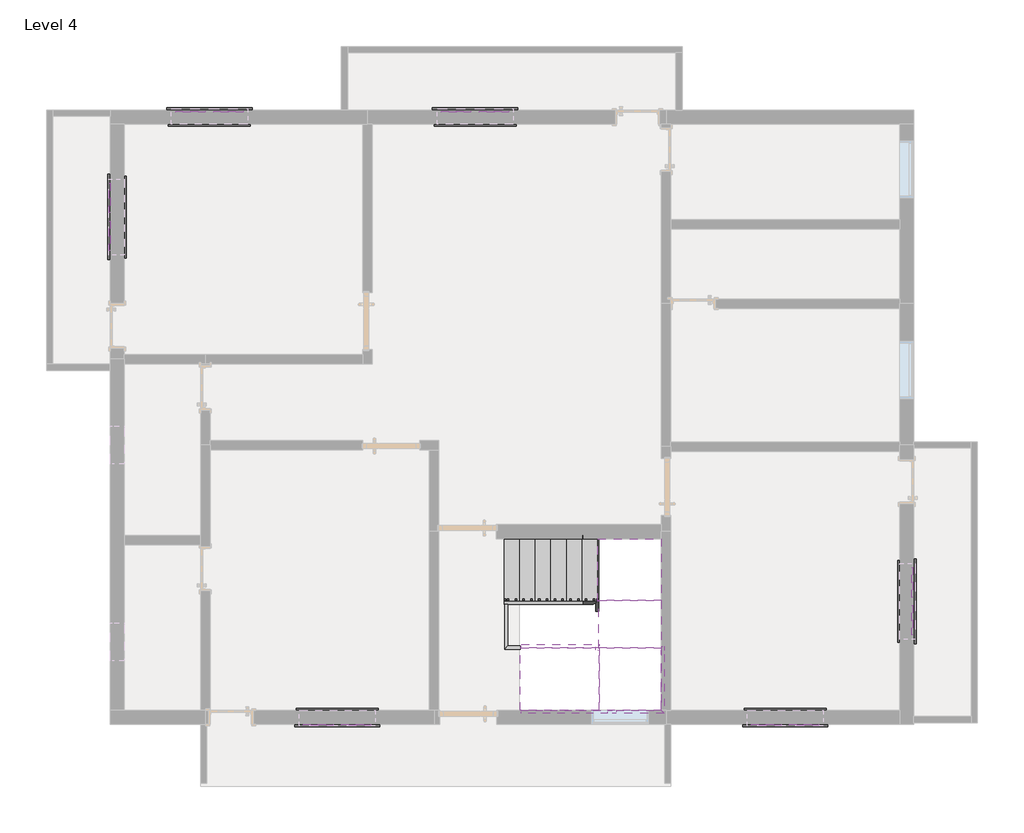
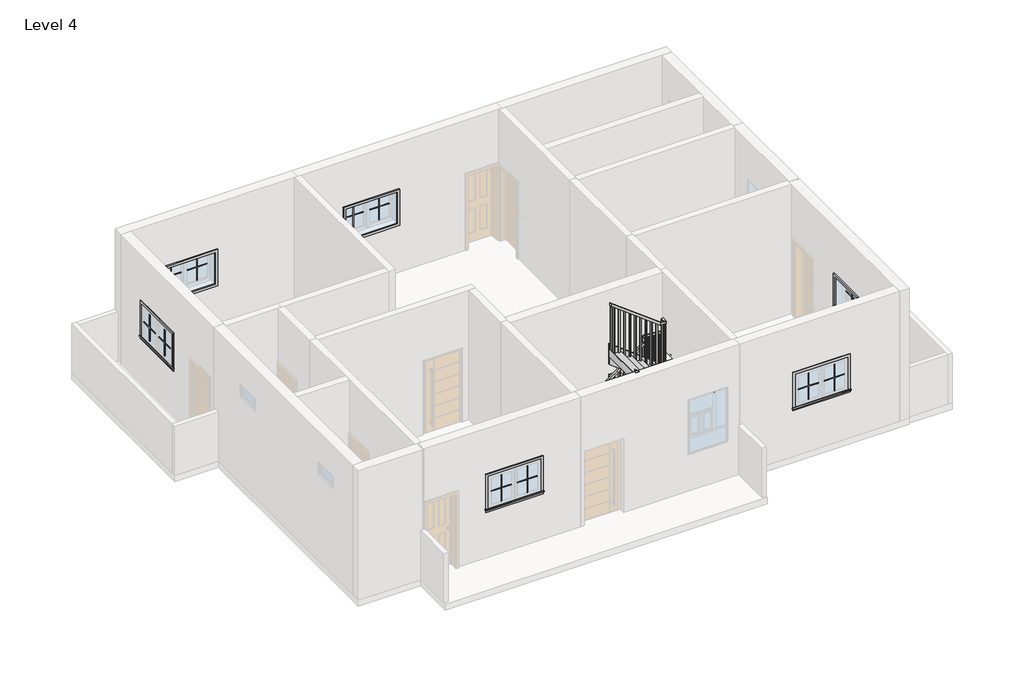
# One storey, part 3 of 3: 24 proxies, 11 members, 3 stair flights, 2 railings, 2 slabs.
"""IFC4 building model written with IfcOpenShell, lengths in millimetres."""

from ifc_helpers import new_model, si_unit, frame, origin, place, context, project, spatial, polyline, outline, extrude, faceted_brep, transform, mapped, element, save
from components import m_muntin_pattern_2x2_m_muntin_pattern_2x2_8d9e5da3, m_muntin_pattern_2x2_m_muntin_pattern_2x2_32a0f80e, m_trim_window_exterior_flat_with_sill_3a557199, m_trim_window_interior_flat_picture_frame_580345df, non_monolithic_landing_cef648f3, non_monolithic_landing_62522cc9, stair_flight_50mm_tread_13mm_riser_d6021486, stair_flight_50mm_tread_13mm_riser_ddd89fd2, stair_flight_50mm_tread_13mm_riser_ab5ce904

model = new_model("IFC4")

# Units and contexts
model_context = context("Model", 3, world=origin())
ifc_project = project(units=[si_unit("LENGTHUNIT", "METRE", prefix="MILLI")], contexts=[model_context])

# Site, building, storey
site = spatial("IfcSite", under=ifc_project)
building = spatial("IfcBuilding", under=site)
storey = spatial("IfcBuildingStorey", under=building, Name="Level 4", Elevation=9601.2)

# Proxies
placement = place(None, origin())
m_muntin_pattern_2x2_m_muntin_pattern_2x2_shape = m_muntin_pattern_2x2_m_muntin_pattern_2x2_8d9e5da3(model_context)
element("IfcBuildingElementProxy", 1, Name="M_Muntin Pattern_2x2 : M_Muntin Pattern_2x2", ObjectType="M_Muntin Pattern_2x2 : M_Muntin Pattern_2x2", at=placement, inside=storey, context=model_context, shape_type="MappedRepresentation", body=[
    mapped(m_muntin_pattern_2x2_m_muntin_pattern_2x2_shape, transform((-14356.7669909, -4470.2368509, 10890.25), x_axis=(-1.0, 0.0, 0.0), y_axis=(0.0, -1.0, 0.0), z_axis=(0.0, 0.0, 1.0))),
])
element("IfcBuildingElementProxy", 2, Name="M_Muntin Pattern_2x2 : M_Muntin Pattern_2x2", ObjectType="M_Muntin Pattern_2x2 : M_Muntin Pattern_2x2", at=placement, inside=storey, context=model_context, shape_type="MappedRepresentation", body=[
    mapped(m_muntin_pattern_2x2_m_muntin_pattern_2x2_shape, transform((-17007.0919909, 5340.5131491, 10890.25), x_axis=(1.0, 0.0, 0.0), y_axis=(0.0, 1.0, 0.0), z_axis=(0.0, 0.0, 1.0))),
])
element("IfcBuildingElementProxy", 3, Name="M_Muntin Pattern_2x2 : M_Muntin Pattern_2x2", ObjectType="M_Muntin Pattern_2x2 : M_Muntin Pattern_2x2", at=placement, inside=storey, context=model_context, shape_type="MappedRepresentation", body=[
    mapped(m_muntin_pattern_2x2_m_muntin_pattern_2x2_shape, transform((-18281.8544909, 3334.7006491, 10890.25), x_axis=(0.0, 1.0, 0.0), y_axis=(-1.0, 0.0, 0.0), z_axis=(0.0, 0.0, 1.0))),
])
element("IfcBuildingElementProxy", 4, Name="M_Muntin Pattern_2x2 : M_Muntin Pattern_2x2", ObjectType="M_Muntin Pattern_2x2 : M_Muntin Pattern_2x2", at=placement, inside=storey, context=model_context, shape_type="MappedRepresentation", body=[
    mapped(m_muntin_pattern_2x2_m_muntin_pattern_2x2_shape, transform((-12757.3544909, 5340.5131491, 10890.25), x_axis=(1.0, 0.0, 0.0), y_axis=(0.0, 1.0, 0.0), z_axis=(0.0, 0.0, 1.0))),
])
element("IfcBuildingElementProxy", 5, Name="M_Muntin Pattern_2x2 : M_Muntin Pattern_2x2", ObjectType="M_Muntin Pattern_2x2 : M_Muntin Pattern_2x2", at=placement, inside=storey, context=model_context, shape_type="MappedRepresentation", body=[
    mapped(m_muntin_pattern_2x2_m_muntin_pattern_2x2_shape, transform((-5448.5044909, -2207.2493509, 10890.25), x_axis=(0.0, -1.0, 0.0), y_axis=(1.0, 0.0, 0.0), z_axis=(0.0, 0.0, 1.0))),
])
element("IfcBuildingElementProxy", 6, Name="M_Muntin Pattern_2x2 : M_Muntin Pattern_2x2", ObjectType="M_Muntin Pattern_2x2 : M_Muntin Pattern_2x2", at=placement, inside=storey, context=model_context, shape_type="MappedRepresentation", body=[
    mapped(m_muntin_pattern_2x2_m_muntin_pattern_2x2_shape, transform((-7193.1669909, -4470.2368509, 10890.25), x_axis=(-1.0, 0.0, 0.0), y_axis=(0.0, -1.0, 0.0), z_axis=(0.0, 0.0, 1.0))),
])
m_muntin_pattern_2x2_m_muntin_pattern_2x2_2_shape = m_muntin_pattern_2x2_m_muntin_pattern_2x2_32a0f80e(model_context)
element("IfcBuildingElementProxy", 7, Name="M_Muntin Pattern_2x2 : M_Muntin Pattern_2x2", ObjectType="M_Muntin Pattern_2x2 : M_Muntin Pattern_2x2", at=placement, inside=storey, context=model_context, shape_type="MappedRepresentation", body=[
    mapped(m_muntin_pattern_2x2_m_muntin_pattern_2x2_2_shape, transform((-14963.1919909, -4470.2368509, 10890.25), x_axis=(1.0, 0.0, 0.0), y_axis=(0.0, 1.0, 0.0), z_axis=(0.0, 0.0, 1.0))),
])
element("IfcBuildingElementProxy", 8, Name="M_Muntin Pattern_2x2 : M_Muntin Pattern_2x2", ObjectType="M_Muntin Pattern_2x2 : M_Muntin Pattern_2x2", at=placement, inside=storey, context=model_context, shape_type="MappedRepresentation", body=[
    mapped(m_muntin_pattern_2x2_m_muntin_pattern_2x2_2_shape, transform((-16400.6669909, 5340.5131491, 10890.25), x_axis=(-1.0, 0.0, 0.0), y_axis=(0.0, -1.0, 0.0), z_axis=(0.0, 0.0, 1.0))),
])
element("IfcBuildingElementProxy", 9, Name="M_Muntin Pattern_2x2 : M_Muntin Pattern_2x2", ObjectType="M_Muntin Pattern_2x2 : M_Muntin Pattern_2x2", at=placement, inside=storey, context=model_context, shape_type="MappedRepresentation", body=[
    mapped(m_muntin_pattern_2x2_m_muntin_pattern_2x2_2_shape, transform((-18281.8544909, 3941.1256491, 10890.25), x_axis=(0.0, -1.0, 0.0), y_axis=(1.0, 0.0, 0.0), z_axis=(0.0, 0.0, 1.0))),
])
element("IfcBuildingElementProxy", 10, Name="M_Muntin Pattern_2x2 : M_Muntin Pattern_2x2", ObjectType="M_Muntin Pattern_2x2 : M_Muntin Pattern_2x2", at=placement, inside=storey, context=model_context, shape_type="MappedRepresentation", body=[
    mapped(m_muntin_pattern_2x2_m_muntin_pattern_2x2_2_shape, transform((-12150.9294909, 5340.5131491, 10890.25), x_axis=(-1.0, 0.0, 0.0), y_axis=(0.0, -1.0, 0.0), z_axis=(0.0, 0.0, 1.0))),
])
element("IfcBuildingElementProxy", 11, Name="M_Muntin Pattern_2x2 : M_Muntin Pattern_2x2", ObjectType="M_Muntin Pattern_2x2 : M_Muntin Pattern_2x2", at=placement, inside=storey, context=model_context, shape_type="MappedRepresentation", body=[
    mapped(m_muntin_pattern_2x2_m_muntin_pattern_2x2_2_shape, transform((-5448.5044909, -2813.6743509, 10890.25), x_axis=(0.0, 1.0, 0.0), y_axis=(-1.0, 0.0, 0.0), z_axis=(0.0, 0.0, 1.0))),
])
element("IfcBuildingElementProxy", 12, Name="M_Muntin Pattern_2x2 : M_Muntin Pattern_2x2", ObjectType="M_Muntin Pattern_2x2 : M_Muntin Pattern_2x2", at=placement, inside=storey, context=model_context, shape_type="MappedRepresentation", body=[
    mapped(m_muntin_pattern_2x2_m_muntin_pattern_2x2_2_shape, transform((-7799.5919909, -4470.2368509, 10890.25), x_axis=(1.0, 0.0, 0.0), y_axis=(0.0, 1.0, 0.0), z_axis=(0.0, 0.0, 1.0))),
])
m_trim_window_exterior_flat_with_sill_shape = m_trim_window_exterior_flat_with_sill_3a557199(model_context)
element("IfcBuildingElementProxy", 13, Name="M_Trim-Window-Exterior-Flat : with Sill", ObjectType="M_Trim-Window-Exterior-Flat : with Sill", at=placement, inside=storey, context=model_context, shape_type="MappedRepresentation", body=[
    mapped(m_trim_window_exterior_flat_with_sill_shape, transform((-14659.9794909, -4479.7618509, 11620.4), x_axis=(1.0, 0.0, 0.0), y_axis=(0.0, 0.0, 1.0), z_axis=(0.0, -1.0, 0.0))),
])
element("IfcBuildingElementProxy", 14, Name="M_Trim-Window-Exterior-Flat : with Sill", ObjectType="M_Trim-Window-Exterior-Flat : with Sill", at=placement, inside=storey, context=model_context, shape_type="MappedRepresentation", body=[
    mapped(m_trim_window_exterior_flat_with_sill_shape, transform((-16703.8794909, 5350.0381491, 11620.4), x_axis=(-1.0, 0.0, 0.0), y_axis=(0.0, 0.0, 1.0), z_axis=(0.0, 1.0, 0.0))),
])
element("IfcBuildingElementProxy", 15, Name="M_Trim-Window-Exterior-Flat : with Sill", ObjectType="M_Trim-Window-Exterior-Flat : with Sill", at=placement, inside=storey, context=model_context, shape_type="MappedRepresentation", body=[
    mapped(m_trim_window_exterior_flat_with_sill_shape, transform((-18291.3794909, 3637.9131491, 11620.4), x_axis=(0.0, -1.0, 0.0), y_axis=(0.0, 0.0, 1.0), z_axis=(-1.0, 0.0, 0.0))),
])
element("IfcBuildingElementProxy", 16, Name="M_Trim-Window-Exterior-Flat : with Sill", ObjectType="M_Trim-Window-Exterior-Flat : with Sill", at=placement, inside=storey, context=model_context, shape_type="MappedRepresentation", body=[
    mapped(m_trim_window_exterior_flat_with_sill_shape, transform((-12454.1419909, 5350.0381491, 11620.4), x_axis=(-1.0, 0.0, 0.0), y_axis=(0.0, 0.0, 1.0), z_axis=(0.0, 1.0, 0.0))),
])
element("IfcBuildingElementProxy", 17, Name="M_Trim-Window-Exterior-Flat : with Sill", ObjectType="M_Trim-Window-Exterior-Flat : with Sill", at=placement, inside=storey, context=model_context, shape_type="MappedRepresentation", body=[
    mapped(m_trim_window_exterior_flat_with_sill_shape, transform((-5438.9794909, -2510.4618509, 11620.4), x_axis=(0.0, 1.0, 0.0), y_axis=(0.0, 0.0, 1.0), z_axis=(1.0, 0.0, 0.0))),
])
element("IfcBuildingElementProxy", 18, Name="M_Trim-Window-Exterior-Flat : with Sill", ObjectType="M_Trim-Window-Exterior-Flat : with Sill", at=placement, inside=storey, context=model_context, shape_type="MappedRepresentation", body=[
    mapped(m_trim_window_exterior_flat_with_sill_shape, transform((-7496.3794909, -4479.7618509, 11620.4), x_axis=(1.0, 0.0, 0.0), y_axis=(0.0, 0.0, 1.0), z_axis=(0.0, -1.0, 0.0))),
])
m_trim_window_interior_flat_picture_frame_shape = m_trim_window_interior_flat_picture_frame_580345df(model_context)
element("IfcBuildingElementProxy", 19, Name="M_Trim-Window-Interior-Flat : Picture Frame", ObjectType="M_Trim-Window-Interior-Flat : Picture Frame", at=placement, inside=storey, context=model_context, shape_type="MappedRepresentation", body=[
    mapped(m_trim_window_interior_flat_picture_frame_shape, transform((-14659.9794909, -4251.1618509, 11620.4), x_axis=(-1.0, 0.0, 0.0), y_axis=(0.0, 0.0, 1.0), z_axis=(0.0, 1.0, 0.0))),
])
element("IfcBuildingElementProxy", 20, Name="M_Trim-Window-Interior-Flat : Picture Frame", ObjectType="M_Trim-Window-Interior-Flat : Picture Frame", at=placement, inside=storey, context=model_context, shape_type="MappedRepresentation", body=[
    mapped(m_trim_window_interior_flat_picture_frame_shape, transform((-16703.8794909, 5121.4381491, 11620.4), x_axis=(1.0, 0.0, 0.0), y_axis=(0.0, 0.0, 1.0), z_axis=(0.0, -1.0, 0.0))),
])
element("IfcBuildingElementProxy", 21, Name="M_Trim-Window-Interior-Flat : Picture Frame", ObjectType="M_Trim-Window-Interior-Flat : Picture Frame", at=placement, inside=storey, context=model_context, shape_type="MappedRepresentation", body=[
    mapped(m_trim_window_interior_flat_picture_frame_shape, transform((-18062.7794909, 3637.9131491, 11620.4), x_axis=(0.0, 1.0, 0.0), y_axis=(0.0, 0.0, 1.0), z_axis=(1.0, 0.0, 0.0))),
])
element("IfcBuildingElementProxy", 22, Name="M_Trim-Window-Interior-Flat : Picture Frame", ObjectType="M_Trim-Window-Interior-Flat : Picture Frame", at=placement, inside=storey, context=model_context, shape_type="MappedRepresentation", body=[
    mapped(m_trim_window_interior_flat_picture_frame_shape, transform((-12454.1419909, 5121.4381491, 11620.4), x_axis=(1.0, 0.0, 0.0), y_axis=(0.0, 0.0, 1.0), z_axis=(0.0, -1.0, 0.0))),
])
element("IfcBuildingElementProxy", 23, Name="M_Trim-Window-Interior-Flat : Picture Frame", ObjectType="M_Trim-Window-Interior-Flat : Picture Frame", at=placement, inside=storey, context=model_context, shape_type="MappedRepresentation", body=[
    mapped(m_trim_window_interior_flat_picture_frame_shape, transform((-5667.5794909, -2510.4618509, 11620.4), x_axis=(0.0, -1.0, 0.0), y_axis=(0.0, 0.0, 1.0), z_axis=(-1.0, 0.0, 0.0))),
])
element("IfcBuildingElementProxy", 24, Name="M_Trim-Window-Interior-Flat : Picture Frame", ObjectType="M_Trim-Window-Interior-Flat : Picture Frame", at=placement, inside=storey, context=model_context, shape_type="MappedRepresentation", body=[
    mapped(m_trim_window_interior_flat_picture_frame_shape, transform((-7496.3794909, -4251.1618509, 11620.4), x_axis=(-1.0, 0.0, 0.0), y_axis=(0.0, 0.0, 1.0), z_axis=(0.0, 1.0, 0.0))),
])

# Members
element("IfcMember", 25, ObjectType="Stringer - 50mm Width", at=placement, inside=storey, context=model_context, shape_type="SweptSolid", body=[
    extrude(outline(polyline([(9854.7429417, -11992.1794909), (9601.2, -11992.1794909), (9601.2, -11663.9259909), (10569.0117647, -10378.7116427), (10969.0117647, -10512.4761733), (9854.7429417, -11992.1794909)])), frame((0.0, -1507.9618509, 0.0), z_axis=(0.0, 1.0, 0.0), x_axis=(0.0, 0.0, 1.0)), (0.0, 0.0, 1.0), 50.0),
])
element("IfcMember", 26, ObjectType="Stringer - 50mm Width", at=placement, inside=storey, context=model_context, shape_type="Brep", body=[
    faceted_brep([(-11992.1794909, -2557.9876321, 9601.2), (-11992.1794909, -2507.9876321, 9601.2), (-11663.9259909, -2507.9876321, 9601.2), (-11663.9259909, -2557.9876321, 9601.2), (-11992.1794909, -2557.9876321, 9854.7429417), (-10569.4898929, -2557.9876321, 10425.349009), (-10569.4898929, -2557.9876321, 10926.0784216), (-10492.1794909, -2507.9876321, 10483.5664703), (-10492.1794909, -2507.9876321, 10969.0117647), (-10512.4761733, -2521.1143795, 10969.0117647), (-11992.1794909, -2507.9876321, 9854.7429417), (-10512.4761733, -2507.9876321, 10969.0117647)], [[[0, 1, 2, 3]], [[4, 0, 3, 5, 6]], [[6, 5, 7, 8, 9]], [[2, 7, 5, 3]], [[1, 10, 11, 8, 7, 2]], [[11, 9, 8]], [[10, 4, 6, 9, 11]], [[4, 10, 1, 0]]]),
])
element("IfcMember", 27, ObjectType="Stringer - 50mm Width", at=placement, inside=storey, context=model_context, shape_type="SweptSolid", body=[
    extrude(outline(polyline([(-2228.2651685, 10969.0117647), (-2362.029699, 10569.0117647), (-3362.029699, 11322.0470588), (-3228.2651685, 11722.0470588), (-2228.2651685, 10969.0117647)])), frame((-9477.5794909, 0.0, 0.0), z_axis=(1.0, 0.0, 0.0), x_axis=(0.0, 1.0, 0.0)), (0.0, 0.0, 1.0), 50.0),
])
element("IfcMember", 28, ObjectType="Stringer - 50mm Width", at=placement, inside=storey, context=model_context, shape_type="Brep", body=[
    faceted_brep([(-10527.6052721, -3234.9066499, 11722.0470588), (-10527.6052721, -3234.9066499, 11226.3189161), (-10477.6052721, -3248.5618509, 11236.6017644), (-10477.6052721, -3248.5618509, 11722.0470588), (-10477.6052721, -3228.2651685, 11722.0470588), (-10527.6052721, -3228.2651685, 11722.0470588), (-10477.6052721, -2498.5618509, 11172.5547064), (-10527.6052721, -2530.8990259, 11196.9057405), (-10477.6052721, -2498.5618509, 10671.8252938), (-10527.6052721, -2530.8990259, 10696.1763279)], [[[0, 1, 2, 3]], [[4, 5, 0, 3]], [[6, 7, 5, 4]], [[7, 6, 8, 9]], [[7, 9, 1, 0, 5]], [[8, 6, 4, 3, 2]], [[9, 8, 2, 1]]]),
])
element("IfcMember", 29, ObjectType="Stringer - 50mm Width", at=placement, inside=storey, context=model_context, shape_type="Brep", body=[
    faceted_brep([(-9477.5794909, -2228.2651685, 10969.0117647), (-9427.5794909, -2228.2651685, 10969.0117647), (-9427.5794909, -1457.9618509, 10969.0117647), (-9477.5794909, -1507.9618509, 10969.0117647), (-9477.5794909, -2362.029699, 10569.0117647), (-9477.5794909, -1507.9618509, 10569.0117647), (-9427.5794909, -2362.029699, 10569.0117647), (-9427.5794909, -1457.9618509, 10569.0117647)], [[[0, 1, 2, 3]], [[4, 0, 3, 5]], [[6, 4, 5, 7]], [[1, 6, 7, 2]], [[1, 0, 4, 6]], [[2, 7, 5, 3]]]),
])
element("IfcMember", 30, ObjectType="Stringer - 50mm Width", at=placement, inside=storey, context=model_context, shape_type="Brep", body=[
    faceted_brep([(-9477.5794909, -1507.9618509, 10969.0117647), (-9427.5794909, -1457.9618509, 10969.0117647), (-10512.4761733, -1457.9618509, 10969.0117647), (-10512.4761733, -1507.9618509, 10969.0117647), (-9477.5794909, -1507.9618509, 10569.0117647), (-10378.7116427, -1507.9618509, 10569.0117647), (-9427.5794909, -1457.9618509, 10569.0117647), (-10378.7116427, -1457.9618509, 10569.0117647)], [[[0, 1, 2, 3]], [[4, 0, 3, 5]], [[6, 4, 5, 7]], [[1, 6, 7, 2]], [[1, 0, 4, 6]], [[2, 7, 5, 3]]]),
])
element("IfcMember", 31, ObjectType="Stringer - 50mm Width", at=placement, inside=storey, context=model_context, shape_type="SweptSolid", body=[
    extrude(outline(polyline([(11322.0470588, -10331.6473391), (11722.0470588, -10197.8828085), (12866.8841182, -11718.1794909), (12366.1547056, -11718.1794909), (11322.0470588, -10331.6473391)])), frame((0.0, -4301.1618509, 0.0), z_axis=(0.0, 1.0, 0.0), x_axis=(0.0, 0.0, 1.0)), (0.0, 0.0, 1.0), 50.0),
])
element("IfcMember", 32, ObjectType="Stringer - 50mm Width", at=placement, inside=storey, context=model_context, shape_type="SweptSolid", body=[
    extrude(outline(polyline([(11424.8605879, -10468.1794909), (11925.5900005, -10468.1794909), (12866.8841182, -11718.1794909), (12366.1547056, -11718.1794909), (11424.8605879, -10468.1794909)])), frame((0.0, -3251.1360696, 0.0), z_axis=(0.0, 1.0, 0.0), x_axis=(0.0, 0.0, 1.0)), (0.0, 0.0, 1.0), 50.0),
])
element("IfcMember", 33, ObjectType="Stringer - 50mm Width", at=placement, inside=storey, context=model_context, shape_type="Brep", body=[
    faceted_brep([(-10197.8828085, -4251.1618509, 11722.0470588), (-10197.8828085, -4301.1618509, 11722.0470588), (-9427.5794909, -4301.1618509, 11722.0470588), (-9477.5794909, -4251.1618509, 11722.0470588), (-10331.6473391, -4251.1618509, 11322.0470588), (-9477.5794909, -4251.1618509, 11322.0470588), (-10331.6473391, -4301.1618509, 11322.0470588), (-9427.5794909, -4301.1618509, 11322.0470588)], [[[0, 1, 2, 3]], [[4, 0, 3, 5]], [[6, 4, 5, 7]], [[1, 6, 7, 2]], [[1, 0, 4, 6]], [[2, 7, 5, 3]]]),
])
element("IfcMember", 34, ObjectType="Stringer - 50mm Width", at=placement, inside=storey, context=model_context, shape_type="Brep", body=[
    faceted_brep([(-9477.5794909, -4251.1618509, 11722.0470588), (-9427.5794909, -4301.1618509, 11722.0470588), (-9427.5794909, -3228.2651685, 11722.0470588), (-9477.5794909, -3228.2651685, 11722.0470588), (-9477.5794909, -4251.1618509, 11322.0470588), (-9477.5794909, -3362.029699, 11322.0470588), (-9427.5794909, -4301.1618509, 11322.0470588), (-9427.5794909, -3362.029699, 11322.0470588)], [[[0, 1, 2, 3]], [[4, 0, 3, 5]], [[6, 4, 5, 7]], [[1, 6, 7, 2]], [[1, 0, 4, 6]], [[2, 7, 5, 3]]]),
])
element("IfcMember", 35, ObjectType="Stringer - 50mm Width", at=placement, inside=storey, context=model_context, shape_type="SweptSolid", body=[
    extrude(outline(polyline([(-10527.6052721, -3286.7377652), (-10527.6052721, -3234.9066499), (-10468.1794909, -3251.1360696), (-10468.1794909, -3302.9671849), (-10527.6052721, -3286.7377652)])), frame((0.0, 0.0, 11322.0470588), z_axis=(0.0, 0.0, 1.0), x_axis=(1.0, 0.0, 0.0)), (0.0, 0.0, 1.0), 400.0),
])

# Railings
element("IfcRailing", 36, ObjectType="1100mm", at=placement, inside=storey, context=model_context, shape_type="SolidModel", body=[
    faceted_brep([(-11992.1794909, -2457.5876321, 10889.4588235), (-11992.1794909, -2457.5876321, 10826.867647), (-11992.1794909, -2507.5876321, 10826.867647), (-11992.1794909, -2507.5876321, 10889.4588235), (-10506.1686883, -2457.5876321, 12008.4774053), (-10493.1861187, -2507.5876321, 12018.2537384), (-10475.1839648, -2507.5876321, 11969.2188191), (-10488.1665344, -2457.5876321, 11959.442486)], [[[0, 1, 2, 3]], [[4, 5, 6, 7]], [[1, 0, 4, 7]], [[2, 1, 7, 6]], [[3, 2, 6, 5]], [[0, 3, 5, 4]]]),
    faceted_brep([(-10507.8033465, -2458.0701724, 12019.0117647), (-10492.6871017, -2448.2938394, 11969.0117647), (-10476.4352157, -2497.3287587, 11969.0117647), (-10491.5514605, -2507.1050918, 12019.0117647), (-10486.7741604, -2444.469683, 12019.0117647), (-10459.6209288, -2486.4542279, 12019.0117647), (-10417.6363839, -2459.3009964, 11969.0117647), (-10444.7896154, -2417.3164514, 11969.0117647)], [[[0, 1, 2, 3]], [[4, 5, 6, 7]], [[1, 0, 4, 7]], [[2, 1, 7, 6]], [[3, 2, 6, 5]], [[0, 3, 5, 4]]]),
    faceted_brep([(-10486.7741604, -2444.469683, 12019.0117647), (-10444.7896154, -2417.3164514, 11969.0117647), (-10417.6363839, -2459.3009964, 11969.0117647), (-10459.6209288, -2486.4542279, 12019.0117647), (-10486.7741604, -2444.469683, 12144.524782), (-10459.6209288, -2486.4542279, 12123.5833848), (-10417.6363839, -2459.3009964, 12137.1270973), (-10444.7896154, -2417.3164514, 12158.0684945)], [[[0, 1, 2, 3]], [[4, 5, 6, 7]], [[1, 0, 4, 7]], [[2, 1, 7, 6]], [[3, 2, 6, 5]], [[0, 3, 5, 4]]]),
    faceted_brep([(-10427.2052721, -2426.8853397, 12153.2956456), (-10427.2052721, -2476.8853397, 12128.3562337), (-10477.2052721, -2476.8853397, 12128.3562337), (-10477.2052721, -2426.8853397, 12153.2956456), (-10427.2052721, -3176.5360696, 12717.8091035), (-10427.2052721, -3226.5360696, 12692.8696916), (-10477.2052721, -3226.5360696, 12692.8696916), (-10477.2052721, -3176.5360696, 12717.8091035), (-10427.2052721, -3176.5360696, 13023.5802613), (-10427.2052721, -3226.5360696, 12973.5802613), (-10477.2052721, -3226.5360696, 12973.5802613), (-10477.2052721, -3176.5360696, 13023.5802613), (-10427.2052721, -3301.5360696, 13023.5802613), (-10427.2052721, -3301.5360696, 12973.5802613), (-10477.2052721, -3251.5360696, 12973.5802613), (-10477.2052721, -3251.5360696, 13023.5802613), (-10552.2052721, -3301.5360696, 13023.5802613), (-10568.9258385, -3301.5360696, 12973.5802613), (-10568.9258385, -3251.5360696, 12973.5802613), (-10552.2052721, -3251.5360696, 13023.5802613), (-11718.1794909, -3301.5360696, 13901.6), (-11718.1794909, -3251.5360696, 13901.6), (-11718.1794909, -3251.5360696, 13839.0088234), (-11718.1794909, -3301.5360696, 13839.0088234)], [[[0, 1, 2, 3]], [[1, 0, 4, 5]], [[2, 1, 5, 6]], [[3, 2, 6, 7]], [[0, 3, 7, 4]], [[5, 4, 8, 9]], [[6, 5, 9, 10]], [[7, 6, 10, 11]], [[4, 7, 11, 8]], [[9, 8, 12, 13]], [[10, 9, 13, 14]], [[11, 10, 14, 15]], [[8, 11, 15, 12]], [[13, 12, 16, 17]], [[14, 13, 17, 18]], [[15, 14, 18, 19]], [[12, 15, 19, 16]], [[20, 21, 22, 23]], [[17, 16, 20, 23]], [[18, 17, 23, 22]], [[19, 18, 22, 21]], [[16, 19, 21, 20]]]),
    extrude(outline(polyline([(12613.3411765, -11627.2052721), (13770.5020258, -11627.2052721), (13789.3279082, -11652.2052721), (12613.3411765, -11652.2052721), (12613.3411765, -11627.2052721)])), frame((0.0, -3289.0360696, 0.0), z_axis=(0.0, 1.0, 0.0), x_axis=(0.0, 0.0, 1.0)), (0.0, 0.0, 1.0), 25.0),
    extrude(outline(polyline([(12613.3411765, -11502.2052721), (13676.3726141, -11502.2052721), (13695.1984964, -11527.2052721), (12613.3411765, -11527.2052721), (12613.3411765, -11502.2052721)])), frame((0.0, -3289.0360696, 0.0), z_axis=(0.0, 1.0, 0.0), x_axis=(0.0, 0.0, 1.0)), (0.0, 0.0, 1.0), 25.0),
    extrude(outline(polyline([(12425.0823529, -11377.2052721), (13582.2432023, -11377.2052721), (13601.0690847, -11402.2052721), (12425.0823529, -11402.2052721), (12425.0823529, -11377.2052721)])), frame((0.0, -3289.0360696, 0.0), z_axis=(0.0, 1.0, 0.0), x_axis=(0.0, 0.0, 1.0)), (0.0, 0.0, 1.0), 25.0),
    extrude(outline(polyline([(12425.0823529, -11252.2052721), (13488.1137906, -11252.2052721), (13506.9396729, -11277.2052721), (12425.0823529, -11277.2052721), (12425.0823529, -11252.2052721)])), frame((0.0, -3289.0360696, 0.0), z_axis=(0.0, 1.0, 0.0), x_axis=(0.0, 0.0, 1.0)), (0.0, 0.0, 1.0), 25.0),
    extrude(outline(polyline([(12236.8235294, -11127.2052721), (13393.9843788, -11127.2052721), (13412.8102611, -11152.2052721), (12236.8235294, -11152.2052721), (12236.8235294, -11127.2052721)])), frame((0.0, -3289.0360696, 0.0), z_axis=(0.0, 1.0, 0.0), x_axis=(0.0, 0.0, 1.0)), (0.0, 0.0, 1.0), 25.0),
    extrude(outline(polyline([(12236.8235294, -11002.2052721), (13299.854967, -11002.2052721), (13318.6808494, -11027.2052721), (12236.8235294, -11027.2052721), (12236.8235294, -11002.2052721)])), frame((0.0, -3289.0360696, 0.0), z_axis=(0.0, 1.0, 0.0), x_axis=(0.0, 0.0, 1.0)), (0.0, 0.0, 1.0), 25.0),
    extrude(outline(polyline([(12048.5647059, -10877.2052721), (13205.7255553, -10877.2052721), (13224.5514376, -10902.2052721), (12048.5647059, -10902.2052721), (12048.5647059, -10877.2052721)])), frame((0.0, -3289.0360696, 0.0), z_axis=(0.0, 1.0, 0.0), x_axis=(0.0, 0.0, 1.0)), (0.0, 0.0, 1.0), 25.0),
    extrude(outline(polyline([(12048.5647059, -10752.2052721), (13111.5961435, -10752.2052721), (13130.4220258, -10777.2052721), (12048.5647059, -10777.2052721), (12048.5647059, -10752.2052721)])), frame((0.0, -3289.0360696, 0.0), z_axis=(0.0, 1.0, 0.0), x_axis=(0.0, 0.0, 1.0)), (0.0, 0.0, 1.0), 25.0),
    extrude(outline(polyline([(11860.3058824, -10627.2052721), (13017.4667317, -10627.2052721), (13036.2926141, -10652.2052721), (11860.3058824, -10652.2052721), (11860.3058824, -10627.2052721)])), frame((0.0, -3289.0360696, 0.0), z_axis=(0.0, 1.0, 0.0), x_axis=(0.0, 0.0, 1.0)), (0.0, 0.0, 1.0), 25.0),
    extrude(outline(polyline([(-10502.2052721, -3264.0360696), (-10502.2052721, -3289.0360696), (-10527.2052721, -3289.0360696), (-10527.2052721, -3264.0360696), (-10502.2052721, -3264.0360696)])), frame((0.0, 0.0, 11860.3058824), z_axis=(0.0, 0.0, 1.0), x_axis=(1.0, 0.0, 0.0)), (0.0, 0.0, 1.0), 1113.2743789),
    extrude(outline(polyline([(-10464.7052721, -3251.8853397), (-10439.7052721, -3251.8853397), (-10439.7052721, -3276.8853397), (-10464.7052721, -3276.8853397), (-10464.7052721, -3251.8853397)])), frame((0.0, 0.0, 11672.0470588), z_axis=(0.0, 0.0, 1.0), x_axis=(1.0, 0.0, 0.0)), (0.0, 0.0, 1.0), 1301.5332024),
    extrude(outline(polyline([(-3126.8853397, 12617.8291749), (-3126.8853397, 11483.7882353), (-3151.8853397, 11483.7882353), (-3151.8853397, 12636.6550572), (-3126.8853397, 12617.8291749)])), frame((-10464.7052721, 0.0, 0.0), z_axis=(1.0, 0.0, 0.0), x_axis=(0.0, 1.0, 0.0)), (0.0, 0.0, 1.0), 25.0),
    extrude(outline(polyline([(-3001.8853397, 12523.6997631), (-3001.8853397, 11483.7882353), (-3026.8853397, 11483.7882353), (-3026.8853397, 12542.5256455), (-3001.8853397, 12523.6997631)])), frame((-10464.7052721, 0.0, 0.0), z_axis=(1.0, 0.0, 0.0), x_axis=(0.0, 1.0, 0.0)), (0.0, 0.0, 1.0), 25.0),
    extrude(outline(polyline([(-2876.8853397, 12429.5703513), (-2876.8853397, 11295.5294118), (-2901.8853397, 11295.5294118), (-2901.8853397, 12448.3962337), (-2876.8853397, 12429.5703513)])), frame((-10464.7052721, 0.0, 0.0), z_axis=(1.0, 0.0, 0.0), x_axis=(0.0, 1.0, 0.0)), (0.0, 0.0, 1.0), 25.0),
    extrude(outline(polyline([(-2751.8853397, 12335.4409396), (-2751.8853397, 11295.5294118), (-2776.8853397, 11295.5294118), (-2776.8853397, 12354.2668219), (-2751.8853397, 12335.4409396)])), frame((-10464.7052721, 0.0, 0.0), z_axis=(1.0, 0.0, 0.0), x_axis=(0.0, 1.0, 0.0)), (0.0, 0.0, 1.0), 25.0),
    extrude(outline(polyline([(-2626.8853397, 12241.3115278), (-2626.8853397, 11107.2705882), (-2651.8853397, 11107.2705882), (-2651.8853397, 12260.1374102), (-2626.8853397, 12241.3115278)])), frame((-10464.7052721, 0.0, 0.0), z_axis=(1.0, 0.0, 0.0), x_axis=(0.0, 1.0, 0.0)), (0.0, 0.0, 1.0), 25.0),
    extrude(outline(polyline([(-2501.8853397, 12147.182116), (-2501.8853397, 11107.2705882), (-2526.8853397, 11107.2705882), (-2526.8853397, 12166.0079984), (-2501.8853397, 12147.182116)])), frame((-10464.7052721, 0.0, 0.0), z_axis=(1.0, 0.0, 0.0), x_axis=(0.0, 1.0, 0.0)), (0.0, 0.0, 1.0), 25.0),
    extrude(outline(polyline([(11899.9429411, -10567.1794909), (10730.7529412, -10567.1794909), (10730.7529412, -10542.1794909), (11918.7688234, -10542.1794909), (11899.9429411, -10567.1794909)])), frame((0.0, -2495.0876321, 0.0), z_axis=(0.0, 1.0, 0.0), x_axis=(0.0, 0.0, 1.0)), (0.0, 0.0, 1.0), 25.0),
    extrude(outline(polyline([(11805.8135293, -10692.1794909), (10730.7529412, -10692.1794909), (10730.7529412, -10667.1794909), (11824.6394117, -10667.1794909), (11805.8135293, -10692.1794909)])), frame((0.0, -2495.0876321, 0.0), z_axis=(0.0, 1.0, 0.0), x_axis=(0.0, 0.0, 1.0)), (0.0, 0.0, 1.0), 25.0),
    extrude(outline(polyline([(11711.6841175, -10817.1794909), (10542.4941176, -10817.1794909), (10542.4941176, -10792.1794909), (11730.5099999, -10792.1794909), (11711.6841175, -10817.1794909)])), frame((0.0, -2495.0876321, 0.0), z_axis=(0.0, 1.0, 0.0), x_axis=(0.0, 0.0, 1.0)), (0.0, 0.0, 1.0), 25.0),
    extrude(outline(polyline([(11617.5547058, -10942.1794909), (10542.4941176, -10942.1794909), (10542.4941176, -10917.1794909), (11636.3805881, -10917.1794909), (11617.5547058, -10942.1794909)])), frame((0.0, -2495.0876321, 0.0), z_axis=(0.0, 1.0, 0.0), x_axis=(0.0, 0.0, 1.0)), (0.0, 0.0, 1.0), 25.0),
    extrude(outline(polyline([(11523.425294, -11067.1794909), (10354.2352941, -11067.1794909), (10354.2352941, -11042.1794909), (11542.2511764, -11042.1794909), (11523.425294, -11067.1794909)])), frame((0.0, -2495.0876321, 0.0), z_axis=(0.0, 1.0, 0.0), x_axis=(0.0, 0.0, 1.0)), (0.0, 0.0, 1.0), 25.0),
    extrude(outline(polyline([(11429.2958822, -11192.1794909), (10354.2352941, -11192.1794909), (10354.2352941, -11167.1794909), (11448.1217646, -11167.1794909), (11429.2958822, -11192.1794909)])), frame((0.0, -2495.0876321, 0.0), z_axis=(0.0, 1.0, 0.0), x_axis=(0.0, 0.0, 1.0)), (0.0, 0.0, 1.0), 25.0),
    extrude(outline(polyline([(11335.1664705, -11317.1794909), (10165.9764706, -11317.1794909), (10165.9764706, -11292.1794909), (11353.9923528, -11292.1794909), (11335.1664705, -11317.1794909)])), frame((0.0, -2495.0876321, 0.0), z_axis=(0.0, 1.0, 0.0), x_axis=(0.0, 0.0, 1.0)), (0.0, 0.0, 1.0), 25.0),
    extrude(outline(polyline([(11241.0370587, -11442.1794909), (10165.9764706, -11442.1794909), (10165.9764706, -11417.1794909), (11259.8629411, -11417.1794909), (11241.0370587, -11442.1794909)])), frame((0.0, -2495.0876321, 0.0), z_axis=(0.0, 1.0, 0.0), x_axis=(0.0, 0.0, 1.0)), (0.0, 0.0, 1.0), 25.0),
    extrude(outline(polyline([(11146.907647, -11567.1794909), (9977.7176471, -11567.1794909), (9977.7176471, -11542.1794909), (11165.7335293, -11542.1794909), (11146.907647, -11567.1794909)])), frame((0.0, -2495.0876321, 0.0), z_axis=(0.0, 1.0, 0.0), x_axis=(0.0, 0.0, 1.0)), (0.0, 0.0, 1.0), 25.0),
    extrude(outline(polyline([(11052.7782352, -11692.1794909), (9977.7176471, -11692.1794909), (9977.7176471, -11667.1794909), (11071.6041175, -11667.1794909), (11052.7782352, -11692.1794909)])), frame((0.0, -2495.0876321, 0.0), z_axis=(0.0, 1.0, 0.0), x_axis=(0.0, 0.0, 1.0)), (0.0, 0.0, 1.0), 25.0),
    extrude(outline(polyline([(10958.6488234, -11817.1794909), (9789.4588235, -11817.1794909), (9789.4588235, -11792.1794909), (10977.4747058, -11792.1794909), (10958.6488234, -11817.1794909)])), frame((0.0, -2495.0876321, 0.0), z_axis=(0.0, 1.0, 0.0), x_axis=(0.0, 0.0, 1.0)), (0.0, 0.0, 1.0), 25.0),
    extrude(outline(polyline([(10864.5194117, -11942.1794909), (9789.4588235, -11942.1794909), (9789.4588235, -11917.1794909), (10883.345294, -11917.1794909), (10864.5194117, -11942.1794909)])), frame((0.0, -2495.0876321, 0.0), z_axis=(0.0, 1.0, 0.0), x_axis=(0.0, 0.0, 1.0)), (0.0, 0.0, 1.0), 25.0),
    extrude(outline(polyline([(-10464.7052721, -3264.0360696), (-10439.7052721, -3264.0360696), (-10439.7052721, -3289.0360696), (-10464.7052721, -3289.0360696), (-10464.7052721, -3264.0360696)])), frame((0.0, 0.0, 11672.0470588), z_axis=(0.0, 0.0, 1.0), x_axis=(1.0, 0.0, 0.0)), (0.0, 0.0, 1.0), 1301.5332024),
    extrude(outline(polyline([(-10455.9131005, -2469.1697838), (-10469.4897163, -2448.1775113), (-10448.4974438, -2434.6008955), (-10434.920828, -2455.593168), (-10455.9131005, -2469.1697838)])), frame((0.0, 0.0, 10919.0117647), z_axis=(0.0, 0.0, 1.0), x_axis=(1.0, 0.0, 0.0)), (0.0, 0.0, 1.0), 1050.0),
    extrude(outline(polyline([(11941.3614541, -10512.1774035), (10730.7529412, -10512.1774035), (10730.7529412, -10487.1774035), (11960.1873365, -10487.1774035), (11941.3614541, -10512.1774035)])), frame((0.0, -2495.0876321, 0.0), z_axis=(0.0, 1.0, 0.0), x_axis=(0.0, 0.0, 1.0)), (0.0, 0.0, 1.0), 25.0),
    extrude(outline(polyline([(12613.3411765, -11693.1794909), (13820.1829411, -11693.1794909), (13839.0088234, -11718.1794909), (12613.3411765, -11718.1794909), (12613.3411765, -11693.1794909)])), frame((0.0, -3289.0360696, 0.0), z_axis=(0.0, 1.0, 0.0), x_axis=(0.0, 0.0, 1.0)), (0.0, 0.0, 1.0), 25.0),
    extrude(outline(polyline([(10826.867647, -11992.1794909), (9789.4588235, -11992.1794909), (9789.4588235, -11967.1794909), (10845.6935293, -11967.1794909), (10826.867647, -11992.1794909)])), frame((0.0, -2495.0876321, 0.0), z_axis=(0.0, 1.0, 0.0), x_axis=(0.0, 0.0, 1.0)), (0.0, 0.0, 1.0), 25.0),
])
element("IfcRailing", 37, ObjectType="900mm", at=placement, inside=storey, context=model_context, shape_type="SolidModel", body=[
    faceted_brep([(-11730.6794909, -3276.1360696, 10642.6), (-11730.6794909, -3276.1360696, 10592.6), (-11730.6794909, -3226.1360696, 10592.6), (-11730.6794909, -3226.1360696, 10642.6), (-11984.2794909, -3276.1360696, 10642.6), (-11984.2794909, -3276.1360696, 10592.6), (-11934.2794909, -3226.1360696, 10592.6), (-11934.2794909, -3226.1360696, 10642.6), (-11984.2794909, -2557.9876321, 10642.6), (-11934.2794909, -2557.9876321, 10642.6), (-11934.2794909, -2557.9876321, 10592.6), (-11984.2794909, -2557.9876321, 10592.6)], [[[0, 1, 2, 3]], [[1, 0, 4, 5]], [[2, 1, 5, 6]], [[3, 2, 6, 7]], [[0, 3, 7, 4]], [[8, 9, 10, 11]], [[5, 4, 8, 11]], [[6, 5, 11, 10]], [[7, 6, 10, 9]], [[4, 7, 9, 8]]]),
    extrude(outline(polyline([(-11949.2794909, -2711.1360696), (-11969.2794909, -2711.1360696), (-11969.2794909, -2691.1360696), (-11949.2794909, -2691.1360696), (-11949.2794909, -2711.1360696)])), frame((0.0, 0.0, 9601.2), z_axis=(0.0, 0.0, 1.0), x_axis=(1.0, 0.0, 0.0)), (0.0, 0.0, 1.0), 991.4),
    extrude(outline(polyline([(-11949.2794909, -2986.1360696), (-11969.2794909, -2986.1360696), (-11969.2794909, -2966.1360696), (-11949.2794909, -2966.1360696), (-11949.2794909, -2986.1360696)])), frame((0.0, 0.0, 9601.2), z_axis=(0.0, 0.0, 1.0), x_axis=(1.0, 0.0, 0.0)), (0.0, 0.0, 1.0), 991.4),
    extrude(outline(polyline([(-11949.2794909, -3241.1360696), (-11949.2794909, -3261.1360696), (-11969.2794909, -3261.1360696), (-11969.2794909, -3241.1360696), (-11949.2794909, -3241.1360696)])), frame((0.0, 0.0, 9601.2), z_axis=(0.0, 0.0, 1.0), x_axis=(1.0, 0.0, 0.0)), (0.0, 0.0, 1.0), 991.4),
    extrude(outline(polyline([(-11949.2794909, -2577.9876321), (-11969.2794909, -2577.9876321), (-11969.2794909, -2557.9876321), (-11949.2794909, -2557.9876321), (-11949.2794909, -2577.9876321)])), frame((0.0, 0.0, 9601.2), z_axis=(0.0, 0.0, 1.0), x_axis=(1.0, 0.0, 0.0)), (0.0, 0.0, 1.0), 991.4),
    extrude(outline(polyline([(-11730.6794909, -3241.1360696), (-11730.6794909, -3261.1360696), (-11750.6794909, -3261.1360696), (-11750.6794909, -3241.1360696), (-11730.6794909, -3241.1360696)])), frame((0.0, 0.0, 9601.2), z_axis=(0.0, 0.0, 1.0), x_axis=(1.0, 0.0, 0.0)), (0.0, 0.0, 1.0), 991.4),
])

# Slabs
non_monolithic_landing_shape = non_monolithic_landing_cef648f3(model_context)
element("IfcSlab", 38, ObjectType="Non-Monolithic Landing", at=placement, inside=storey, context=model_context, shape_type="MappedRepresentation", body=[
    mapped(non_monolithic_landing_shape, transform((0.0, 0.0, 0.0), x_axis=(1.0, 0.0, 0.0), y_axis=(0.0, 1.0, 0.0), z_axis=(0.0, 0.0, 1.0))),
])
non_monolithic_landing_2_shape = non_monolithic_landing_62522cc9(model_context)
element("IfcSlab", 39, ObjectType="Non-Monolithic Landing", at=placement, inside=storey, context=model_context, shape_type="MappedRepresentation", body=[
    mapped(non_monolithic_landing_2_shape, transform((0.0, 0.0, 0.0), x_axis=(1.0, 0.0, 0.0), y_axis=(0.0, 1.0, 0.0), z_axis=(0.0, 0.0, 1.0))),
])

# Stair flights
stair_flight_50mm_tread_13mm_riser_shape = stair_flight_50mm_tread_13mm_riser_d6021486(model_context)
element("IfcStairFlight", 40, ObjectType="50mm Tread 13mm Riser", at=placement, inside=storey, context=model_context, shape_type="MappedRepresentation", body=[
    mapped(stair_flight_50mm_tread_13mm_riser_shape, transform((0.0, 0.0, 0.0), x_axis=(1.0, 0.0, 0.0), y_axis=(0.0, 1.0, 0.0), z_axis=(0.0, 0.0, 1.0))),
])
stair_flight_50mm_tread_13mm_riser_2_shape = stair_flight_50mm_tread_13mm_riser_ddd89fd2(model_context)
element("IfcStairFlight", 41, ObjectType="50mm Tread 13mm Riser", at=placement, inside=storey, context=model_context, shape_type="MappedRepresentation", body=[
    mapped(stair_flight_50mm_tread_13mm_riser_2_shape, transform((0.0, 0.0, 0.0), x_axis=(1.0, 0.0, 0.0), y_axis=(0.0, 1.0, 0.0), z_axis=(0.0, 0.0, 1.0))),
])
stair_flight_50mm_tread_13mm_riser_3_shape = stair_flight_50mm_tread_13mm_riser_ab5ce904(model_context)
element("IfcStairFlight", 42, ObjectType="50mm Tread 13mm Riser", at=placement, inside=storey, context=model_context, shape_type="MappedRepresentation", body=[
    mapped(stair_flight_50mm_tread_13mm_riser_3_shape, transform((0.0, 0.0, 0.0), x_axis=(1.0, 0.0, 0.0), y_axis=(0.0, 1.0, 0.0), z_axis=(0.0, 0.0, 1.0))),
])

save(model, "model.ifc")

# Revit data of these elements
# Type "M_Muntin Pattern_2x2 : M_Muntin Pattern_2x2"
#   Width [instance default] = 3' - 11.24409"
#   Thickness = 0' - 0 1/2"
#   Height [instance default] = 3' - 11.24409"
#   Distance = 0' - 0 3/4"
#   Interior Material [instance default] = none
#   Exterior Material [instance default] = none
#   Default Elevation = 0
# Type "M_Trim-Window-Exterior-Flat : with Sill"
#   Trim Width = 0' - 2.3622"
#   Trim Thickness_Picture Frame = 0' - 1.1811"
#   Trim Thickness_with Sill = 0' - 0 3/4"
#   Sill Thickness = 0' - 1.1811"
#   Opening Width [instance default] = 1' - 11.62205"
#   Opening Height [instance default] = 2' - 11.43307"
#   Default Elevation = 3' - 11.24409"
#   Sill = yes
#   Picture Frame = no
#   Trim Material [instance default] = none
# Type "M_Trim-Window-Interior-Flat : Picture Frame"
#   Trim Thickness_Picture Frame = 0' - 1.1811"
#   Trim Width = 0' - 2.3622"
#   Trim Thickness_with Sill = 0' - 0.7874"
#   Sill Thickness = 0' - 1.1811"
#   Opening Width [instance default] = 1' - 11.62205"
#   Opening Height [instance default] = 2' - 11.43307"
#   Default Elevation = 3' - 11.24409"
#   Sill = no
#   Picture Frame = yes
#   Trim Material [instance default] = none
# Type "1100mm"
#   built-in parameter 1008612 = 0.019685 (stored number, unit not read)
#   built-in parameter 1008611 = 0.019685 (stored number, unit not read)
#   built-in parameter 1008609 = 0.902231 (stored number, unit not read)
#   built-in parameter 1008604 = 0.19685 (stored number, unit not read)
#   built-in parameter 1008603 = 0.164042 (stored number, unit not read)
#   Railing Height = 3' - 7.30709"
#   built-in parameter 1008630 = 2
#   built-in parameter 1008610 = 2
#   built-in parameter 1008608 = 1
#   built-in parameter 1008618 = M_Baluster - Square : 25mm
# Type "900mm"
#   built-in parameter 1008612 = 0.019685 (stored number, unit not read)
#   built-in parameter 1008611 = 0.019685 (stored number, unit not read)
#   built-in parameter 1008609 = 0.902231 (stored number, unit not read)
#   built-in parameter 1008604 = 0.19685 (stored number, unit not read)
#   built-in parameter 1008603 = 0.164042 (stored number, unit not read)
#   Railing Height = 3' - 5"
#   built-in parameter 1008630 = 2
#   built-in parameter 1008610 = 2
#   built-in parameter 1008608 = 1
#   built-in parameter 1008618 = M_Baluster - Square : 20mm
# Elements 1, 2, 3, 4, 5, 6, 7, 8, 9, 10, 11, 12 (IfcBuildingElementProxy, "M_Muntin Pattern_2x2 : M_Muntin Pattern_2x2")
#   Width = 1' - 6 5/8"
#   Height = 2' - 1.99606"
#   Interior Material = Wood - Stained
#   Exterior Material = Clad - White
#   Phase Created = New Construction
#   Materials on its faces: "Clad - White", "Wood - Stained"
# Elements 13, 14, 15, 16, 17, 18 (IfcBuildingElementProxy, "M_Trim-Window-Exterior-Flat : with Sill")
#   Opening Width = 4' - 0"
#   Opening Height = 2' - 7.49606"
#   Trim Material = Clad - White
#   Phase Created = New Construction
#   Materials on its faces: "Clad - White"
# Elements 19, 20, 21, 22, 23, 24 (IfcBuildingElementProxy, "M_Trim-Window-Interior-Flat : Picture Frame")
#   Opening Width = 4' - 0"
#   Opening Height = 2' - 7.49606"
#   Trim Material = Wood - Stained
#   Phase Created = New Construction
#   Materials on its faces: "Wood - Stained"
# Elements 25, 26, 27, 28, 29, 30, 31, 32, 33, 34, 35 (IfcMember, "Stringer - 50mm Width")
#   Phase Created = New Construction
# Element 36 (IfcRailing, "1100mm")
#   Phase Created = New Construction
# Element 37 (IfcRailing, "900mm")
#   Phase Created = New Construction
# Elements 38, 39 (IfcSlab, "Non-Monolithic Landing")
#   Phase Created = New Construction
# Elements 40, 41, 42 (IfcStairFlight, "50mm Tread 13mm Riser")
#   Phase Created = New Construction
# Materials
#   "Clad - White": class "Wood", colour RGB 242 242 238, transparency 0, Cost = 0
#   "Wood - Stained": class "Wood", colour RGB 224 178 126, transparency 0, Cost = 0
